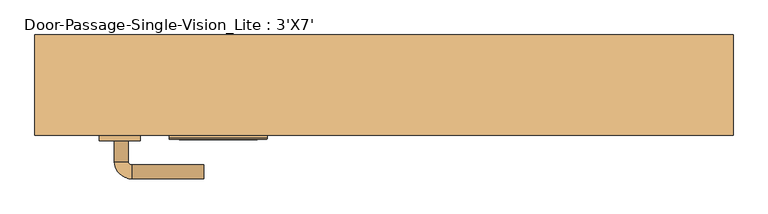
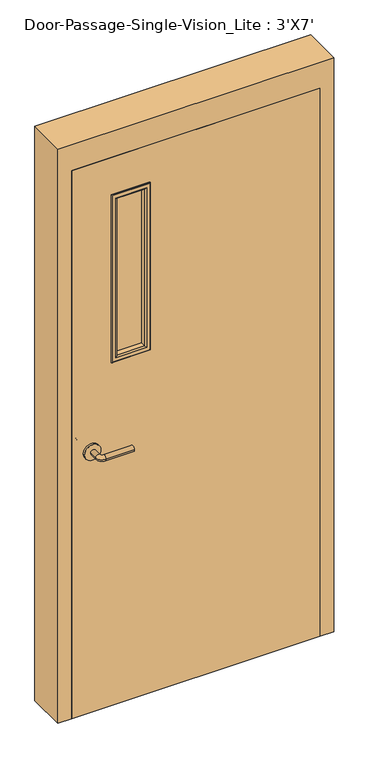
"""IFC4 building model written with IfcOpenShell, lengths in millimetres: door geometry, Door-Passage-Single-Vision_Lite : 3'X7'."""

from ifc_helpers import new_model, si_unit, point, frame, frame_2d, origin, place, context, project, spatial, polyline, circle_curve, ellipse_curve, trimmed, segment, composite_curve, outline, extrude, faceted_brep, source, transform, mapped, element, save
from ifc_brep_helpers import plane_surface, cylinder_surface, revolved_surface, advanced_brep


def door_passage_single_vision_lite_3_x7_38248cdf(model_context):
    return source(origin(), model_context, "Body", "SolidModel", [
        advanced_brep(
        [(-392.190625, 14.35, 1016.0), (-372.190625, 14.35, 1016.0), (-392.190625, 44.35, 1016.0), (-372.190625, 44.35, 1016.0), (-367.190625, 49.35, 1016.0), (-367.190625, 69.35, 1016.0), (-262.190625, 69.35, 1016.0), (-262.190625, 49.35, 1016.0)],
        [
            (0, 1, circle_curve(frame((-382.190625, 14.35, 1016.0), z_axis=(0.0, -1.0, 0.0), x_axis=(1.0, 0.0, 0.0)), 10.0)),
            (1, 0, circle_curve(frame((-382.190625, 14.35, 1016.0), z_axis=(0.0, -1.0, 0.0), x_axis=(1.0, 0.0, 0.0)), 10.0)),
            (0, 2),
            (2, 3, circle_curve(frame((-382.190625, 44.35, 1016.0), z_axis=(0.0, -1.0, 0.0), x_axis=(1.0, 0.0, 0.0)), 10.0)),
            (3, 1),
            (3, 2, circle_curve(frame((-382.190625, 44.35, 1016.0), z_axis=(0.0, -1.0, 0.0), x_axis=(1.0, 0.0, 0.0)), 10.0)),
            (4, 3, circle_curve(frame((-367.190625, 44.35, 1016.0), z_axis=(0.0, 0.0, 1.0), x_axis=(-1.0, 0.0, 0.0)), 5.0)),
            (2, 5, circle_curve(frame((-367.190625, 44.35, 1016.0), z_axis=(0.0, 0.0, -1.0), x_axis=(-1.0, 0.0, 0.0)), 25.0)),
            (5, 4, circle_curve(frame((-367.190625, 59.35, 1016.0), z_axis=(-1.0, 0.0, 0.0), x_axis=(0.0, -1.0, 0.0)), 10.0)),
            (4, 5, circle_curve(frame((-367.190625, 59.35, 1016.0), z_axis=(-1.0, 0.0, 0.0), x_axis=(0.0, -1.0, 0.0)), 10.0)),
            (6, 7, circle_curve(frame((-262.190625, 59.35, 1016.0), z_axis=(1.0, 0.0, 0.0), x_axis=(0.0, -1.0, 0.0)), 10.0)),
            (7, 6, circle_curve(frame((-262.190625, 59.35, 1016.0), z_axis=(1.0, 0.0, 0.0), x_axis=(0.0, -1.0, 0.0)), 10.0)),
            (5, 6),
            (7, 4),
        ],
        [
            plane_surface(frame((-382.190625, 14.35, 1016.0), z_axis=(0.0, -1.0, 0.0), x_axis=(0.0, 0.0, 1.0))),
            cylinder_surface(frame((-382.190625, 14.35, 1016.0), z_axis=(0.0, -1.0, 0.0), x_axis=(1.0, 0.0, 0.0)), 10.0),
            revolved_surface(trimmed(ellipse_curve(frame((-382.190625, 44.35, 1016.0), z_axis=(0.0, -1.0, 0.0), x_axis=(1.0, 0.0, 0.0)), 10.0, 10.0), [point((-392.190625, 44.35, 1016.0))], [point((-372.190625, 44.35, 1016.0))], True, "CARTESIAN"), (-367.190625, 44.35, 1016.0), (0.0, 0.0, -1.0)),
            revolved_surface(trimmed(ellipse_curve(frame((-382.190625, 44.35, 1016.0), z_axis=(0.0, -1.0, 0.0), x_axis=(1.0, 0.0, 0.0)), 10.0, 10.0), [point((-372.190625, 44.35, 1016.0))], [point((-392.190625, 44.35, 1016.0))], True, "CARTESIAN"), (-367.190625, 44.35, 1016.0), (0.0, 0.0, -1.0)),
            plane_surface(frame((-262.190625, 59.35, 1016.0), z_axis=(1.0, 0.0, 0.0), x_axis=(0.0, 0.0, 1.0))),
            cylinder_surface(frame((-367.190625, 59.35, 1016.0), z_axis=(-1.0, 0.0, 0.0), x_axis=(0.0, -1.0, 0.0)), 10.0),
        ],
        [
            (0, [[1, 2]]),
            (1, [[-1, 3, 4, 5]]),
            (1, [[-2, -5, 6, -3]]),
            (2, [[7, -4, 8, 9]]),
            (3, [[-8, -6, -7, 10]]),
            (4, [[11, 12]]),
            (5, [[-9, 13, -12, 14]]),
            (5, [[-10, -14, -11, -13]]),
        ],
    ),
        extrude(outline(composite_curve([segment(trimmed(circle_curve(frame_2d((1016.0, -384.690625)), 30.0), [point((1016.0, -414.690625))], [point((1016.0, -354.690625))], False, "CARTESIAN"), True, "CONTINUOUS"), segment(trimmed(circle_curve(frame_2d((1016.0, -384.690625)), 30.0), [point((1016.0, -354.690625))], [point((1016.0, -414.690625))], False, "CARTESIAN"), True, "CONTINUOUS")], self_intersect=False)), frame((0.0, 6.35, 0.0), z_axis=(0.0, 1.0, 0.0), x_axis=(0.0, 0.0, 1.0)), (0.0, 0.0, 1.0), 8.0),
        advanced_brep(
        [(-392.190625, -46.1, 1016.0), (-372.190625, -46.1, 1016.0), (-372.190625, -76.1, 1016.0), (-392.190625, -76.1, 1016.0), (-367.190625, -81.1, 1016.0), (-367.190625, -101.1, 1016.0), (-262.190625, -101.1, 1016.0), (-262.190625, -81.1, 1016.0)],
        [
            (0, 1, circle_curve(frame((-382.190625, -46.1, 1016.0), z_axis=(0.0, 1.0, 0.0), x_axis=(1.0, 0.0, 0.0)), 10.0)),
            (1, 0, circle_curve(frame((-382.190625, -46.1, 1016.0), z_axis=(0.0, 1.0, 0.0), x_axis=(1.0, 0.0, 0.0)), 10.0)),
            (1, 2),
            (2, 3, circle_curve(frame((-382.190625, -76.1, 1016.0), z_axis=(0.0, 1.0, 0.0), x_axis=(1.0, 0.0, 0.0)), 10.0)),
            (3, 0),
            (3, 2, circle_curve(frame((-382.190625, -76.1, 1016.0), z_axis=(0.0, 1.0, 0.0), x_axis=(1.0, 0.0, 0.0)), 10.0)),
            (4, 5, circle_curve(frame((-367.190625, -91.1, 1016.0), z_axis=(-1.0, 0.0, 0.0), x_axis=(0.0, 1.0, 0.0)), 10.0)),
            (5, 3, circle_curve(frame((-367.190625, -76.1, 1016.0), z_axis=(0.0, 0.0, -1.0), x_axis=(-1.0, 0.0, 0.0)), 25.0)),
            (2, 4, circle_curve(frame((-367.190625, -76.1, 1016.0), z_axis=(0.0, 0.0, 1.0), x_axis=(-1.0, 0.0, 0.0)), 5.0)),
            (5, 4, circle_curve(frame((-367.190625, -91.1, 1016.0), z_axis=(-1.0, 0.0, 0.0), x_axis=(0.0, 1.0, 0.0)), 10.0)),
            (6, 7, circle_curve(frame((-262.190625, -91.1, 1016.0), z_axis=(1.0, 0.0, 0.0), x_axis=(0.0, 1.0, 0.0)), 10.0)),
            (7, 6, circle_curve(frame((-262.190625, -91.1, 1016.0), z_axis=(1.0, 0.0, 0.0), x_axis=(0.0, 1.0, 0.0)), 10.0)),
            (4, 7),
            (6, 5),
        ],
        [
            plane_surface(frame((-382.190625, -46.1, 1016.0), z_axis=(0.0, 1.0, 0.0), x_axis=(0.0, 0.0, 1.0))),
            cylinder_surface(frame((-382.190625, -46.1, 1016.0), z_axis=(0.0, 1.0, 0.0), x_axis=(1.0, 0.0, 0.0)), 10.0),
            revolved_surface(trimmed(ellipse_curve(frame((-382.190625, -76.1, 1016.0), z_axis=(0.0, -1.0, 0.0), x_axis=(1.0, 0.0, 0.0)), 10.0, 10.0), [point((-392.190625, -76.1, 1016.0))], [point((-372.190625, -76.1, 1016.0))], True, "CARTESIAN"), (-367.190625, -76.1, 1016.0), (0.0, 0.0, -1.0)),
            revolved_surface(trimmed(ellipse_curve(frame((-382.190625, -76.1, 1016.0), z_axis=(0.0, -1.0, 0.0), x_axis=(1.0, 0.0, 0.0)), 10.0, 10.0), [point((-372.190625, -76.1, 1016.0))], [point((-392.190625, -76.1, 1016.0))], True, "CARTESIAN"), (-367.190625, -76.1, 1016.0), (0.0, 0.0, -1.0)),
            plane_surface(frame((-262.190625, -91.1, 1016.0), z_axis=(1.0, 0.0, 0.0), x_axis=(0.0, 0.0, 1.0))),
            cylinder_surface(frame((-367.190625, -91.1, 1016.0), z_axis=(-1.0, 0.0, 0.0), x_axis=(0.0, 1.0, 0.0)), 10.0),
        ],
        [
            (0, [[1, 2]]),
            (1, [[3, 4, 5, -2]]),
            (1, [[-5, 6, -3, -1]]),
            (2, [[7, 8, -4, 9]]),
            (3, [[10, -9, -6, -8]]),
            (4, [[11, 12]]),
            (5, [[13, -11, 14, -7]]),
            (5, [[-14, -12, -13, -10]]),
        ],
    ),
        extrude(outline(composite_curve([segment(trimmed(circle_curve(frame_2d((1016.0, -384.690625)), 30.0), [point((1016.0, -414.690625))], [point((1016.0, -354.690625))], False, "CARTESIAN"), True, "CONTINUOUS"), segment(trimmed(circle_curve(frame_2d((1016.0, -384.690625)), 30.0), [point((1016.0, -354.690625))], [point((1016.0, -414.690625))], False, "CARTESIAN"), True, "CONTINUOUS")], self_intersect=False)), frame((0.0, -46.1, 0.0), z_axis=(0.0, 1.0, 0.0), x_axis=(0.0, 0.0, 1.0)), (0.0, 0.0, 1.0), 8.0),
        extrude(outline(polyline([(2133.6, -457.2), (0.0, -457.2), (0.0, 457.2), (2133.6, 457.2), (2133.6, -457.2)]), holes=[polyline([(1981.2, -304.8), (1981.2, -177.8), (1346.2, -177.8), (1346.2, -304.8), (1981.2, -304.8)])]), frame((0.0, -38.1, 0.0), z_axis=(0.0, 1.0, 0.0), x_axis=(0.0, 0.0, 1.0)), (0.0, 0.0, 1.0), 44.45),
        faceted_brep([(457.2, 11.1125, 0.0), (441.325, 11.1125, 0.0), (441.325, 58.7375, 0.0), (457.2, 58.7375, 0.0), (457.2, 107.95, 0.0), (508.0, 107.95, 0.0), (508.0, -38.1, 0.0), (457.2, -38.1, 0.0), (457.2, -38.1, 2133.6), (457.2, 11.1125, 2133.6), (508.0, -38.1, 2235.2), (-508.0, -38.1, 2235.2), (-508.0, -38.1, 0.0), (-457.2, -38.1, 0.0), (-457.2, -38.1, 2133.6), (508.0, 107.95, 2235.2), (457.2, 107.95, 2133.6), (-457.2, 107.95, 2133.6), (-457.2, 107.95, 0.0), (-508.0, 107.95, 0.0), (-508.0, 107.95, 2235.2), (457.2, 58.7375, 2133.6), (441.325, 58.7375, 2117.725), (-441.325, 58.7375, 2117.725), (-441.325, 58.7375, 0.0), (-457.2, 58.7375, 0.0), (-457.2, 58.7375, 2133.6), (441.325, 11.1125, 2117.725), (-457.2, 11.1125, 2133.6), (-457.2, 11.1125, 0.0), (-441.325, 11.1125, 0.0), (-441.325, 11.1125, 2117.725)], [[[0, 1, 2, 3, 4, 5, 6, 7]], [[7, 8, 9, 0]], [[6, 10, 11, 12, 13, 14, 8, 7]], [[5, 15, 10, 6]], [[4, 16, 17, 18, 19, 20, 15, 5]], [[3, 21, 16, 4]], [[2, 22, 23, 24, 25, 26, 21, 3]], [[1, 27, 22, 2]], [[0, 9, 28, 29, 30, 31, 27, 1]], [[8, 14, 28, 9]], [[16, 21, 26, 17]], [[22, 27, 31, 23]], [[12, 19, 18, 25, 24, 30, 29, 13]], [[13, 29, 28, 14]], [[11, 20, 19, 12]], [[17, 26, 25, 18]], [[23, 31, 30, 24]], [[15, 20, 11, 10]]]),
        extrude(outline(polyline([(-177.8, -12.7), (-177.8, -19.05), (-304.8, -19.05), (-304.8, -12.7), (-177.8, -12.7)])), frame((0.0, 0.0, 1346.2), z_axis=(0.0, 0.0, 1.0), x_axis=(1.0, 0.0, 0.0)), (0.0, 0.0, 1.0), 635.0),
        advanced_brep(
        [(-304.8, -19.05, 1981.2), (-304.8, -19.05, 1346.2), (-304.8, -38.1, 1346.2), (-304.8, -38.1, 1981.2), (-292.8, -39.1, 1969.2), (-292.8, -39.1, 1358.2), (-292.8, -19.05, 1358.2), (-292.8, -19.05, 1969.2), (-297.8, -44.1, 1974.2), (-297.8, -44.1, 1353.2), (-312.8, -42.1, 1989.2), (-312.8, -42.1, 1338.2), (-310.8, -44.1, 1340.2), (-310.8, -44.1, 1987.2), (-312.8, -38.1, 1989.2), (-312.8, -38.1, 1338.2), (-177.8, -19.05, 1346.2), (-177.8, -38.1, 1346.2), (-189.8, -39.1, 1358.2), (-189.8, -19.05, 1358.2), (-184.8, -44.1, 1353.2), (-169.8, -42.1, 1338.2), (-171.8, -44.1, 1340.2), (-169.8, -38.1, 1338.2), (-177.8, -19.05, 1981.2), (-177.8, -38.1, 1981.2), (-189.8, -39.1, 1969.2), (-189.8, -19.05, 1969.2), (-184.8, -44.1, 1974.2), (-169.8, -42.1, 1989.2), (-171.8, -44.1, 1987.2), (-169.8, -38.1, 1989.2)],
        [
            (0, 1),
            (1, 2),
            (2, 3),
            (3, 0),
            (4, 5),
            (5, 6),
            (6, 7),
            (7, 4),
            (8, 9),
            (9, 5, ellipse_curve(frame((-297.8, -39.1, 1353.2), z_axis=(-0.7071067811865475, 0.0, 0.7071067811865475), x_axis=(0.7071067811865474, 0.0, 0.7071067811865476)), 7.0710678, 5.0)),
            (4, 8, ellipse_curve(frame((-297.8, -39.1, 1974.2), z_axis=(-0.7071067811865475, 0.0, -0.7071067811865475), x_axis=(-0.7071067811865474, 0.0, 0.7071067811865476)), 7.0710678, 5.0)),
            (10, 11),
            (11, 12, ellipse_curve(frame((-310.8, -42.1, 1340.2), z_axis=(-0.7071067811865475, 0.0, 0.7071067811865475), x_axis=(0.7071067811865474, 0.0, 0.7071067811865476)), 2.8284271, 2.0)),
            (12, 13),
            (13, 10, ellipse_curve(frame((-310.8, -42.1, 1987.2), z_axis=(-0.7071067811865475, 0.0, -0.7071067811865475), x_axis=(-0.7071067811865474, 0.0, 0.7071067811865476)), 2.8284271, 2.0)),
            (14, 15),
            (15, 11),
            (10, 14),
            (1, 16),
            (16, 17),
            (17, 2),
            (5, 18),
            (18, 19),
            (19, 6),
            (9, 20),
            (20, 18, ellipse_curve(frame((-184.8, -39.1, 1353.2), z_axis=(-0.7071067811865475, 0.0, -0.7071067811865475), x_axis=(-0.7071067811865476, 0.0, 0.7071067811865474)), 7.0710678, 5.0)),
            (11, 21),
            (21, 22, ellipse_curve(frame((-171.8, -42.1, 1340.2), z_axis=(-0.7071067811865475, 0.0, -0.7071067811865475), x_axis=(-0.7071067811865476, 0.0, 0.7071067811865474)), 2.8284271, 2.0)),
            (22, 12),
            (15, 23),
            (23, 21),
            (16, 24),
            (24, 25),
            (25, 17),
            (18, 26),
            (26, 27),
            (27, 19),
            (20, 28),
            (28, 26, ellipse_curve(frame((-184.8, -39.1, 1974.2), z_axis=(0.7071067811865475, 0.0, -0.7071067811865475), x_axis=(-0.7071067811865474, 0.0, -0.7071067811865476)), 7.0710678, 5.0)),
            (21, 29),
            (29, 30, ellipse_curve(frame((-171.8, -42.1, 1987.2), z_axis=(0.7071067811865475, 0.0, -0.7071067811865475), x_axis=(-0.7071067811865474, 0.0, -0.7071067811865476)), 2.8284271, 2.0)),
            (30, 22),
            (23, 31),
            (31, 29),
            (14, 31),
            (25, 3),
            (24, 0),
            (27, 7),
            (26, 4),
            (28, 8),
            (30, 13),
            (29, 10),
        ],
        [
            plane_surface(frame((-304.8, -38.1, 1981.2), z_axis=(-1.0, 0.0, 0.0), x_axis=(0.0, 0.0, -1.0))),
            plane_surface(frame((-292.8, -19.05, 1969.2), z_axis=(1.0, 0.0, 0.0), x_axis=(0.0, 0.0, -1.0))),
            cylinder_surface(frame((-297.8, -39.1, 1981.2), z_axis=(0.0, 0.0, 1.0), x_axis=(-1.0, 0.0, 0.0)), 5.0),
            cylinder_surface(frame((-310.8, -42.1, 1981.2), z_axis=(0.0, 0.0, 1.0), x_axis=(-1.0, 0.0, 0.0)), 2.0),
            plane_surface(frame((-312.8, -42.1, 1989.2), z_axis=(-1.0, 0.0, 0.0), x_axis=(0.0, 0.0, -1.0))),
            plane_surface(frame((-304.8, -38.1, 1346.2), z_axis=(0.0, 0.0, -1.0), x_axis=(1.0, 0.0, 0.0))),
            plane_surface(frame((-292.8, -19.05, 1358.2), z_axis=(0.0, 0.0, 1.0), x_axis=(1.0, 0.0, 0.0))),
            cylinder_surface(frame((-304.8, -39.1, 1353.2), z_axis=(-1.0, 0.0, 0.0), x_axis=(0.0, 0.0, -1.0)), 5.0),
            cylinder_surface(frame((-304.8, -42.1, 1340.2), z_axis=(-1.0, 0.0, 0.0), x_axis=(0.0, 0.0, -1.0)), 2.0),
            plane_surface(frame((-312.8, -42.1, 1338.2), z_axis=(0.0, 0.0, -1.0), x_axis=(1.0, 0.0, 0.0))),
            plane_surface(frame((-177.8, -38.1, 1346.2), z_axis=(1.0, 0.0, 0.0), x_axis=(0.0, 0.0, 1.0))),
            plane_surface(frame((-189.8, -19.05, 1358.2), z_axis=(-1.0, 0.0, 0.0), x_axis=(0.0, 0.0, 1.0))),
            cylinder_surface(frame((-184.8, -39.1, 1346.2), z_axis=(0.0, 0.0, -1.0), x_axis=(1.0, 0.0, 0.0)), 5.0),
            cylinder_surface(frame((-171.8, -42.1, 1346.2), z_axis=(0.0, 0.0, -1.0), x_axis=(1.0, 0.0, 0.0)), 2.0),
            plane_surface(frame((-169.8, -42.1, 1338.2), z_axis=(1.0, 0.0, 0.0), x_axis=(0.0, 0.0, 1.0))),
            plane_surface(frame((-169.8, -38.1, 1989.2), z_axis=(0.0, 1.0, 0.0), x_axis=(-1.0, 0.0, 0.0))),
            plane_surface(frame((-177.8, -38.1, 1981.2), z_axis=(0.0, 0.0, 1.0), x_axis=(-1.0, 0.0, 0.0))),
            plane_surface(frame((-177.8, -19.05, 1981.2), z_axis=(0.0, 1.0, 0.0), x_axis=(-1.0, 0.0, 0.0))),
            plane_surface(frame((-189.8, -19.05, 1969.2), z_axis=(0.0, 0.0, -1.0), x_axis=(-1.0, 0.0, 0.0))),
            cylinder_surface(frame((-177.8, -39.1, 1974.2), z_axis=(1.0, 0.0, 0.0), x_axis=(0.0, 0.0, 1.0)), 5.0),
            plane_surface(frame((-184.8, -44.1, 1974.2), z_axis=(0.0, -1.0, 0.0), x_axis=(-1.0, 0.0, 0.0))),
            cylinder_surface(frame((-177.8, -42.1, 1987.2), z_axis=(1.0, 0.0, 0.0), x_axis=(0.0, 0.0, 1.0)), 2.0),
            plane_surface(frame((-169.8, -42.1, 1989.2), z_axis=(0.0, 0.0, 1.0), x_axis=(-1.0, 0.0, 0.0))),
        ],
        [
            (0, [[1, 2, 3, 4]]),
            (1, [[5, 6, 7, 8]]),
            (2, [[9, 10, -5, 11]]),
            (3, [[12, 13, 14, 15]]),
            (4, [[16, 17, -12, 18]]),
            (5, [[19, 20, 21, -2]]),
            (6, [[22, 23, 24, -6]]),
            (7, [[25, 26, -22, -10]]),
            (8, [[27, 28, 29, -13]]),
            (9, [[30, 31, -27, -17]]),
            (10, [[32, 33, 34, -20]]),
            (11, [[35, 36, 37, -23]]),
            (12, [[38, 39, -35, -26]]),
            (13, [[40, 41, 42, -28]]),
            (14, [[43, 44, -40, -31]]),
            (15, [[-16, 45, -43, -30], [-3, -21, -34, 46]]),
            (16, [[47, -4, -46, -33]]),
            (17, [[-1, -47, -32, -19], [-7, -24, -37, 48]]),
            (18, [[49, -8, -48, -36]]),
            (19, [[50, -11, -49, -39]]),
            (20, [[-14, -29, -42, 51], [-9, -50, -38, -25]]),
            (21, [[52, -15, -51, -41]]),
            (22, [[-45, -18, -52, -44]]),
        ],
    ),
        advanced_brep(
        [(-304.8, -12.7, 1346.2), (-304.8, -12.7, 1981.2), (-304.8, 6.35, 1981.2), (-304.8, 6.35, 1346.2), (-292.8, 7.35, 1358.2), (-292.8, 7.35, 1969.2), (-292.8, -12.7, 1969.2), (-292.8, -12.7, 1358.2), (-297.8, 12.35, 1353.2), (-297.8, 12.35, 1974.2), (-312.8, 10.35, 1338.2), (-312.8, 10.35, 1989.2), (-310.8, 12.35, 1987.2), (-310.8, 12.35, 1340.2), (-312.8, 6.35, 1338.2), (-312.8, 6.35, 1989.2), (-177.8, -12.7, 1981.2), (-177.8, 6.35, 1981.2), (-189.8, 7.35, 1969.2), (-189.8, -12.7, 1969.2), (-184.8, 12.35, 1974.2), (-169.8, 10.35, 1989.2), (-171.8, 12.35, 1987.2), (-169.8, 6.35, 1989.2), (-177.8, -12.7, 1346.2), (-177.8, 6.35, 1346.2), (-189.8, 7.35, 1358.2), (-189.8, -12.7, 1358.2), (-184.8, 12.35, 1353.2), (-169.8, 10.35, 1338.2), (-171.8, 12.35, 1340.2), (-169.8, 6.35, 1338.2)],
        [
            (0, 1),
            (1, 2),
            (2, 3),
            (3, 0),
            (4, 5),
            (5, 6),
            (6, 7),
            (7, 4),
            (8, 9),
            (9, 5, ellipse_curve(frame((-297.8, 7.35, 1974.2), z_axis=(-0.7071067811865475, 0.0, -0.7071067811865475), x_axis=(0.7071067811865474, 0.0, -0.7071067811865476)), 7.0710678, 5.0)),
            (4, 8, ellipse_curve(frame((-297.8, 7.35, 1353.2), z_axis=(-0.7071067811865475, 0.0, 0.7071067811865475), x_axis=(-0.7071067811865474, 0.0, -0.7071067811865476)), 7.0710678, 5.0)),
            (10, 11),
            (11, 12, ellipse_curve(frame((-310.8, 10.35, 1987.2), z_axis=(-0.7071067811865475, 0.0, -0.7071067811865475), x_axis=(0.7071067811865474, 0.0, -0.7071067811865476)), 2.8284271, 2.0)),
            (12, 13),
            (13, 10, ellipse_curve(frame((-310.8, 10.35, 1340.2), z_axis=(-0.7071067811865475, 0.0, 0.7071067811865475), x_axis=(-0.7071067811865474, 0.0, -0.7071067811865476)), 2.8284271, 2.0)),
            (14, 15),
            (15, 11),
            (10, 14),
            (1, 16),
            (16, 17),
            (17, 2),
            (5, 18),
            (18, 19),
            (19, 6),
            (9, 20),
            (20, 18, ellipse_curve(frame((-184.8, 7.35, 1974.2), z_axis=(-0.7071067811865475, 0.0, 0.7071067811865475), x_axis=(-0.7071067811865476, 0.0, -0.7071067811865474)), 7.0710678, 5.0)),
            (11, 21),
            (21, 22, ellipse_curve(frame((-171.8, 10.35, 1987.2), z_axis=(-0.7071067811865475, 0.0, 0.7071067811865475), x_axis=(-0.7071067811865476, 0.0, -0.7071067811865474)), 2.8284271, 2.0)),
            (22, 12),
            (15, 23),
            (23, 21),
            (16, 24),
            (24, 25),
            (25, 17),
            (18, 26),
            (26, 27),
            (27, 19),
            (20, 28),
            (28, 26, ellipse_curve(frame((-184.8, 7.35, 1353.2), z_axis=(0.7071067811865475, 0.0, 0.7071067811865475), x_axis=(-0.7071067811865474, 0.0, 0.7071067811865476)), 7.0710678, 5.0)),
            (21, 29),
            (29, 30, ellipse_curve(frame((-171.8, 10.35, 1340.2), z_axis=(0.7071067811865475, 0.0, 0.7071067811865475), x_axis=(-0.7071067811865474, 0.0, 0.7071067811865476)), 2.8284271, 2.0)),
            (30, 22),
            (23, 31),
            (31, 29),
            (14, 31),
            (25, 3),
            (24, 0),
            (27, 7),
            (26, 4),
            (28, 8),
            (30, 13),
            (29, 10),
        ],
        [
            plane_surface(frame((-304.8, 6.35, 1346.2), z_axis=(-1.0, 0.0, 0.0), x_axis=(0.0, 0.0, 1.0))),
            plane_surface(frame((-292.8, -12.7, 1358.2), z_axis=(1.0, 0.0, 0.0), x_axis=(0.0, 0.0, 1.0))),
            cylinder_surface(frame((-297.8, 7.35, 1346.2), z_axis=(0.0, 0.0, -1.0), x_axis=(-1.0, 0.0, 0.0)), 5.0),
            cylinder_surface(frame((-310.8, 10.35, 1346.2), z_axis=(0.0, 0.0, -1.0), x_axis=(-1.0, 0.0, 0.0)), 2.0),
            plane_surface(frame((-312.8, 10.35, 1338.2), z_axis=(-1.0, 0.0, 0.0), x_axis=(0.0, 0.0, 1.0))),
            plane_surface(frame((-304.8, 6.35, 1981.2), z_axis=(0.0, 0.0, 1.0), x_axis=(1.0, 0.0, 0.0))),
            plane_surface(frame((-292.8, -12.7, 1969.2), z_axis=(0.0, 0.0, -1.0), x_axis=(1.0, 0.0, 0.0))),
            cylinder_surface(frame((-304.8, 7.35, 1974.2), z_axis=(-1.0, 0.0, 0.0), x_axis=(0.0, 0.0, 1.0)), 5.0),
            cylinder_surface(frame((-304.8, 10.35, 1987.2), z_axis=(-1.0, 0.0, 0.0), x_axis=(0.0, 0.0, 1.0)), 2.0),
            plane_surface(frame((-312.8, 10.35, 1989.2), z_axis=(0.0, 0.0, 1.0), x_axis=(1.0, 0.0, 0.0))),
            plane_surface(frame((-177.8, 6.35, 1981.2), z_axis=(1.0, 0.0, 0.0), x_axis=(0.0, 0.0, -1.0))),
            plane_surface(frame((-189.8, -12.7, 1969.2), z_axis=(-1.0, 0.0, 0.0), x_axis=(0.0, 0.0, -1.0))),
            cylinder_surface(frame((-184.8, 7.35, 1981.2), z_axis=(0.0, 0.0, 1.0), x_axis=(1.0, 0.0, 0.0)), 5.0),
            cylinder_surface(frame((-171.8, 10.35, 1981.2), z_axis=(0.0, 0.0, 1.0), x_axis=(1.0, 0.0, 0.0)), 2.0),
            plane_surface(frame((-169.8, 10.35, 1989.2), z_axis=(1.0, 0.0, 0.0), x_axis=(0.0, 0.0, -1.0))),
            plane_surface(frame((-169.8, 6.35, 1338.2), z_axis=(0.0, -1.0, 0.0), x_axis=(-1.0, 0.0, 0.0))),
            plane_surface(frame((-177.8, 6.35, 1346.2), z_axis=(0.0, 0.0, -1.0), x_axis=(-1.0, 0.0, 0.0))),
            plane_surface(frame((-177.8, -12.7, 1346.2), z_axis=(0.0, -1.0, 0.0), x_axis=(-1.0, 0.0, 0.0))),
            plane_surface(frame((-189.8, -12.7, 1358.2), z_axis=(0.0, 0.0, 1.0), x_axis=(-1.0, 0.0, 0.0))),
            cylinder_surface(frame((-177.8, 7.35, 1353.2), z_axis=(1.0, 0.0, 0.0), x_axis=(0.0, 0.0, -1.0)), 5.0),
            plane_surface(frame((-184.8, 12.35, 1353.2), z_axis=(0.0, 1.0, 0.0), x_axis=(-1.0, 0.0, 0.0))),
            cylinder_surface(frame((-177.8, 10.35, 1340.2), z_axis=(1.0, 0.0, 0.0), x_axis=(0.0, 0.0, -1.0)), 2.0),
            plane_surface(frame((-169.8, 10.35, 1338.2), z_axis=(0.0, 0.0, -1.0), x_axis=(-1.0, 0.0, 0.0))),
        ],
        [
            (0, [[1, 2, 3, 4]]),
            (1, [[5, 6, 7, 8]]),
            (2, [[9, 10, -5, 11]]),
            (3, [[12, 13, 14, 15]]),
            (4, [[16, 17, -12, 18]]),
            (5, [[19, 20, 21, -2]]),
            (6, [[22, 23, 24, -6]]),
            (7, [[25, 26, -22, -10]]),
            (8, [[27, 28, 29, -13]]),
            (9, [[30, 31, -27, -17]]),
            (10, [[32, 33, 34, -20]]),
            (11, [[35, 36, 37, -23]]),
            (12, [[38, 39, -35, -26]]),
            (13, [[40, 41, 42, -28]]),
            (14, [[43, 44, -40, -31]]),
            (15, [[-16, 45, -43, -30], [-3, -21, -34, 46]]),
            (16, [[47, -4, -46, -33]]),
            (17, [[-1, -47, -32, -19], [-7, -24, -37, 48]]),
            (18, [[49, -8, -48, -36]]),
            (19, [[50, -11, -49, -39]]),
            (20, [[-14, -29, -42, 51], [-9, -50, -38, -25]]),
            (21, [[52, -15, -51, -41]]),
            (22, [[-45, -18, -52, -44]]),
        ],
    ),
    ])


if __name__ == "__main__":
    model = new_model("IFC4")
    model_context = context("Model", 3, world=origin())
    ifc_project = project(units=[si_unit("LENGTHUNIT", "METRE", prefix="MILLI")], contexts=[model_context])
    site = spatial("IfcSite", under=ifc_project)
    building = spatial("IfcBuilding", under=site)
    placement = place(None, origin())
    door_passage_single_vision_lite_3_x7_shape = door_passage_single_vision_lite_3_x7_38248cdf(model_context)
    element("IfcDoor", 1, ObjectType="Door-Passage-Single-Vision_Lite : 3'X7'", at=placement, inside=building, context=model_context, shape_type="MappedRepresentation", body=[
        mapped(door_passage_single_vision_lite_3_x7_shape, transform((0.0, 0.0, 0.0), x_axis=(1.0, 0.0, 0.0), y_axis=(0.0, 1.0, 0.0), z_axis=(0.0, 0.0, 1.0))),
    ])
    save(model, "model.ifc")

# Revit data of these elements
# Type "Door-Passage-Single-Vision_Lite : 3'X7'"
#   Type Mark = "9"
#   Assembly Code = "B2030100"
#   Analytic Construction = "Wooden"
#   Thickness = 0' - 1 3/4"
#   Thermal Resistance (R) = 2.5876 (h·ft²·°F)/BTU
#   Swing Angle [instance default] = 90.00°
#   Strike Height = 3' - 4"
#   Rough Width [instance default] = 3' - 4"
#   Rough Height [instance default] = 7' - 4"
#   MFOpeningHeight [instance default] = 0' - 4"
#   MFOpeningWidth [instance default] = 0' - 4"
#   Inset Calculate [instance default] = 0' - 4"
#   Masonry Inset [instance default] = 0' - 1"
#   Height = 7' - 0"
#   Width = 3' - 0"
#   Heat Transfer Coefficient (U) = 0.3865 BTU/(h·ft²·°F)
#   Masonry Frame Depth = 0' - 5 3/4"
#   Masonry Frame [instance default] = yes
#   Function = 1
#   Dry Wall Frame [instance default] = no
#   Panel Material = Wood - Birch
#   Glazing = Glass
#   Glass Stop Material = Metal - Paint Finish - Grey
#   Frame Material = Metal - Paint Finish - Grey
#   Door Handle Material = Aluminum
#   Visual Light Transmittance = 0
#   Solar Heat Gain Coefficient = 0
#   Wall Closure = (empty or 0)
# Element 1 (IfcDoor, "Door-Passage-Single-Vision_Lite : 3'X7'")
#   Materials on its faces: "Metal - Paint Finish - Grey", "Aluminum", "Wood - Birch", "Glass"
# Materials
#   "Wood - Birch": class "Wood", colour RGB 166 116 52, transparency 0, Cost = 0
#   "Glass": class "Glass", colour RGB 0 128 192, transparency 0.75, Description = "Soda Lime Glass", Cost = 0
#   "Metal - Paint Finish - Grey": class "Paint", colour RGB 104 104 104, transparency 0, Cost = 0
#   "Aluminum": class "Metal", colour RGB 247 247 247, transparency 0, Description = "Aluminum 6061", Cost = 0
